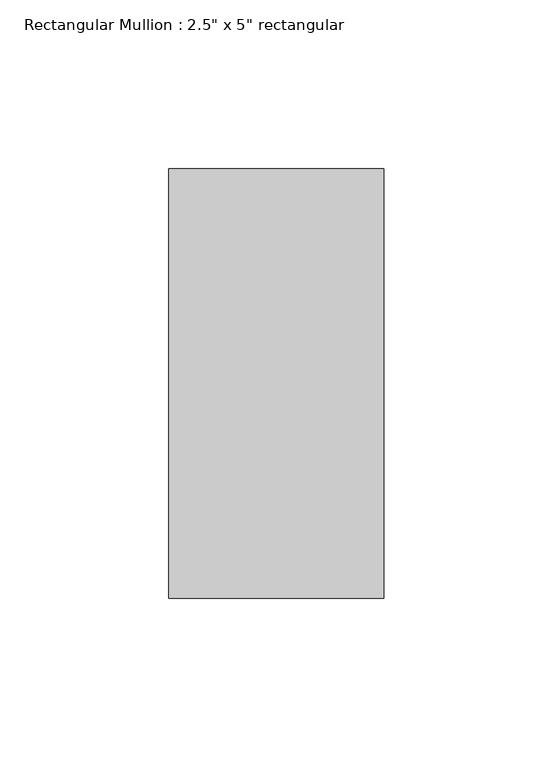
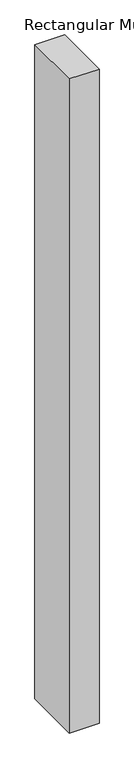
"""IFC4 building model written with IfcOpenShell, lengths in millimetres: member geometry."""

from ifc_helpers import new_model, si_unit, frame, origin, place, context, project, spatial, polyline, outline, extrude, source, transform, mapped, element, save


def member_0bc7eccf(model_context):
    return source(origin(), model_context, "Body", "SweptSolid", [
        extrude(outline(polyline([(0.0, 63.5), (0.0, -63.5), (-63.5, -63.5), (-63.5, 63.5), (0.0, 63.5)])), frame((0.0, 0.0, -1475.7058851), z_axis=(0.0, 0.0, 1.0), x_axis=(1.0, 0.0, 0.0)), (0.0, 0.0, 1.0), 1475.7058851),
    ])


if __name__ == "__main__":
    model = new_model("IFC4")
    model_context = context("Model", 3, world=origin())
    ifc_project = project(units=[si_unit("LENGTHUNIT", "METRE", prefix="MILLI")], contexts=[model_context])
    site = spatial("IfcSite", under=ifc_project)
    building = spatial("IfcBuilding", under=site)
    placement = place(None, origin())
    member_shape = member_0bc7eccf(model_context)
    element("IfcMember", 1, ObjectType="Rectangular Mullion : 2.5\" x 5\" rectangular", at=placement, inside=building, context=model_context, shape_type="MappedRepresentation", body=[
        mapped(member_shape, transform((0.0, 0.0, 0.0), x_axis=(1.0, 0.0, 0.0), y_axis=(0.0, 1.0, 0.0), z_axis=(0.0, 0.0, 1.0))),
    ])
    save(model, "model.ifc")

# Revit data of these elements
# Type "Rectangular Mullion : 2.5\" x 5\" rectangular"
#   built-in parameter 1007304 = 0.416667 (stored number, unit not read)
#   built-in parameter 1007301 = 0.104167 (stored number, unit not read)
#   built-in parameter 1007300 = 0.104167 (stored number, unit not read)
# Element 1 (IfcMember, "Rectangular Mullion : 2.5\" x 5\" rectangular")
#   Materials on its faces: "Aluminum"
# Materials
#   "Aluminum": class "Metal", colour RGB 247 247 247, transparency 0, Description = "Aluminum 6061", Cost = 0
